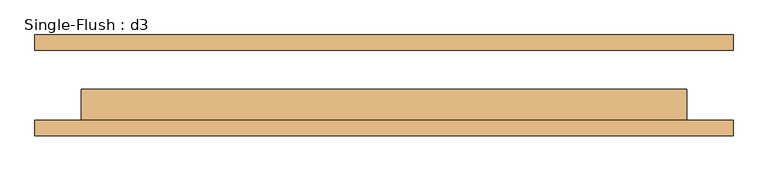
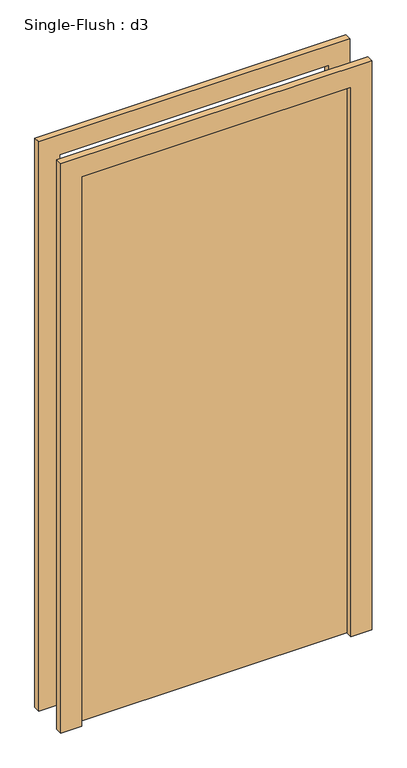
"""IFC4 building model written with IfcOpenShell, lengths in millimetres: door geometry, Single-Flush : d3."""

from ifc_helpers import new_model, si_unit, frame, origin, origin_with_axes, place, context, project, spatial, polyline, outline, extrude, source, transform, mapped, element, save


def single_flush_d3_43e5c869(model_context):
    return source(origin(), model_context, "Body", "SweptSolid", [
        extrude(outline(polyline([(2209.8, -571.5), (0.0, -571.5), (0.0, -495.3), (2133.6, -495.3), (2133.6, 495.3), (0.0, 495.3), (0.0, 571.5), (2209.8, 571.5), (2209.8, -571.5)])), frame((0.0, -82.55, 0.0), z_axis=(0.0, 1.0, 0.0), x_axis=(0.0, 0.0, 1.0)), (0.0, 0.0, 1.0), 25.4),
        extrude(outline(polyline([(2209.8, 571.5), (2209.8, -571.5), (0.0, -571.5), (0.0, -495.3), (2133.6, -495.3), (2133.6, 495.3), (0.0, 495.3), (0.0, 571.5), (2209.8, 571.5)])), frame((0.0, 57.15, 0.0), z_axis=(0.0, 1.0, 0.0), x_axis=(0.0, 0.0, 1.0)), (0.0, 0.0, 1.0), 25.4),
        extrude(outline(polyline([(495.3, -6.35), (495.3, -57.15), (-495.3, -57.15), (-495.3, -6.35), (495.3, -6.35)])), origin_with_axes(), (0.0, 0.0, 1.0), 2133.6),
    ])


if __name__ == "__main__":
    model = new_model("IFC4")
    model_context = context("Model", 3, world=origin())
    ifc_project = project(units=[si_unit("LENGTHUNIT", "METRE", prefix="MILLI")], contexts=[model_context])
    site = spatial("IfcSite", under=ifc_project)
    building = spatial("IfcBuilding", under=site)
    placement = place(None, origin())
    single_flush_d3_shape = single_flush_d3_43e5c869(model_context)
    element("IfcDoor", 1, ObjectType="Single-Flush : d3", at=placement, inside=building, context=model_context, shape_type="MappedRepresentation", body=[
        mapped(single_flush_d3_shape, transform((0.0, 0.0, 0.0), x_axis=(1.0, 0.0, 0.0), y_axis=(0.0, 1.0, 0.0), z_axis=(0.0, 0.0, 1.0))),
    ])
    save(model, "model.ifc")

# Revit data of these elements
# Type "Single-Flush : d3"
#   Type Mark = "10"
#   Construction Type Id = "MDOOR"
#   Assembly Code = "C1020"
#   Analytic Construction = "Metal"
#   Thickness = 0' - 2"
#   Heat Transfer Coefficient (U) = 0.651978 BTU/(h·ft²·°F)
#   Height = 7' - 0"
#   Trim Projection Ext = 0' - 1"
#   Trim Projection Int = 0' - 1"
#   Trim Width = 0' - 3"
#   Width = 3' - 3"
#   Define Thermal Properties by = 1
#   Door Material = Door - Panel
#   Frame Material = Door - Frame
#   Visual Light Transmittance = 0
#   Solar Heat Gain Coefficient = 0
#   Function = (empty or 0)
#   Wall Closure = (empty or 0)
# Element 1 (IfcDoor, "Single-Flush : d3")
#   Materials on its faces: "Door - Frame", "Door - Panel"
# Materials
#   "Door - Panel": class "Wood", colour RGB 210 159 95, transparency 0, Cost = 0
#   "Door - Frame": colour RGB 118 70 51, transparency 0, Cost = 0
